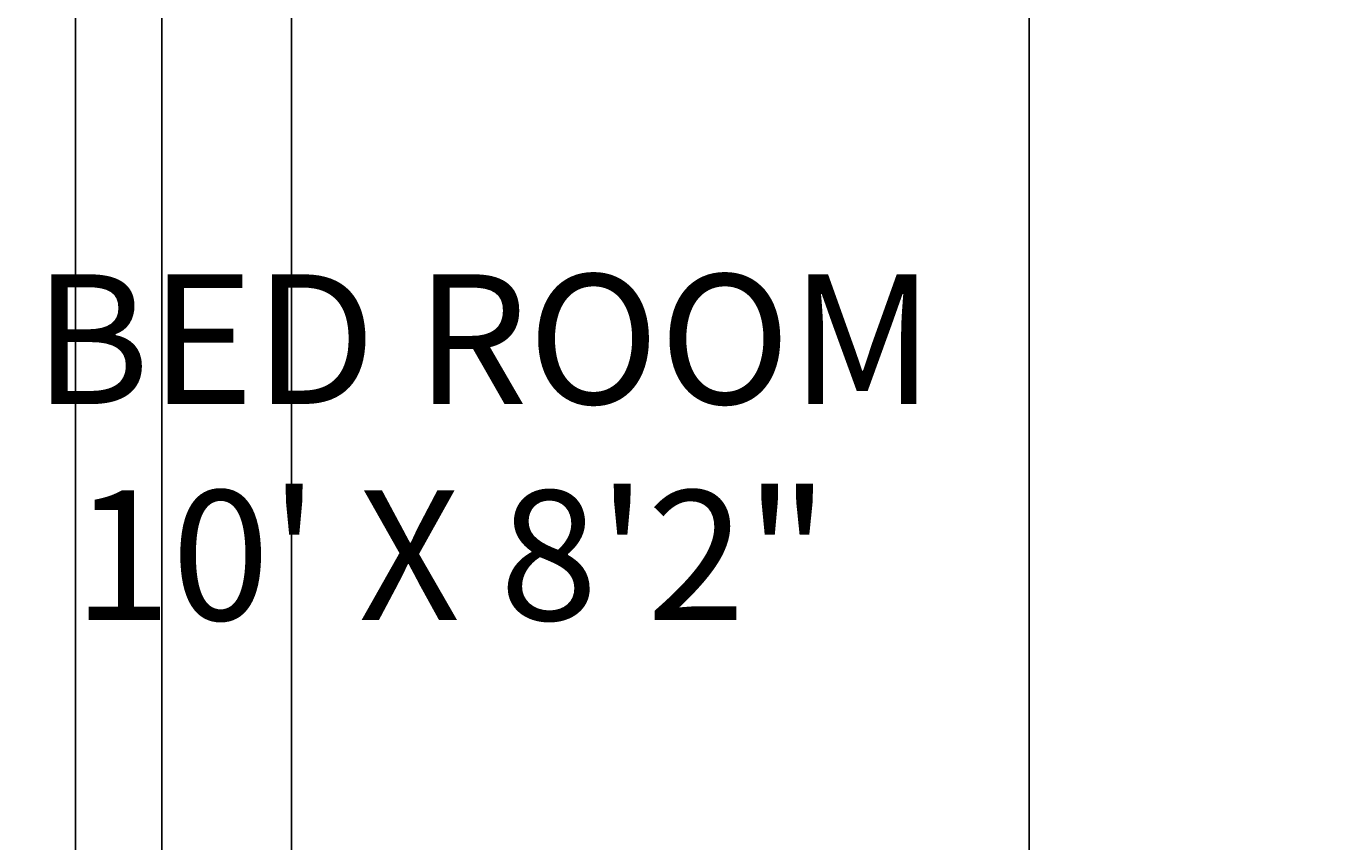
# Model space of a CAD drawing. Units: inches. Extents: x 37 to 824, y -700 to 234.
# Tile 55 of 77: x 204 to 264, y 122 to 160. Entities that reach past the tile are written whole.
import ezdxf

# ---------------------------------------------------------------- set-up
doc = ezdxf.new("R2010")
doc.units = ezdxf.units.IN
doc.header["$MEASUREMENT"] = 0
doc.layers.add('A-ANNO-DIMS', color=2, linetype='Continuous', lineweight=18)
doc.layers.add('A-AREA-IDEN', color=3, linetype='Continuous', lineweight=18)
doc.styles.get("Standard").update_dxf_attribs({"font": 'arial.ttf'})
doc.dimstyles.get("Standard").update_dxf_attribs({"dimtxt": 0.18, "dimasz": 0.18, "dimexe": 0.18, "dimexo": 0.0625, "dimgap": 0.09, "dimtad": 0, "dimtih": 1, "dimtoh": 1, "dimdec": 1, "dimzin": 0, "dimdsep": 46, "dimlunit": 4, "dimtxsty": 'Standard', "dimcen": 0.09, "dimadec": 0, "dimazin": 0, "dimtfac": 1, "dimtdec": 1, "dimtofl": 0, "dimtmove": 0, "dimatfit": 3, "dimfxl": 1, "dimtolj": 1, "dimtzin": 0, "dimarcsym": 0})

# ---------------------------------------------------------------- blocks, each defined once
blk = doc.blocks.new('*D72')
at = {"layer": 'A-ANNO-DIMS', "color": 0, "lineweight": -2, "ltscale": 0.5, "transparency": 16777216}
for p, q in [((170.077, 84.153), (170.077, 234.17)), ((250.19, 84.153), (250.19, 234.17)), ((170.257, 233.99), (209.804, 233.99)), ((250.01, 233.99), (210.463, 233.99))]:
    blk.add_line(p, q, dxfattribs=at)
at = {"layer": 'A-ANNO-DIMS', "color": 0, "ltscale": 0.5, "transparency": 16777216}
for points in [[(170.257, 234.02), (170.257, 233.96), (170.077, 233.99)], [(250.01, 234.02), (250.01, 233.96), (250.19, 233.99)]]:
    blk.add_solid(points, dxfattribs=at)
at = {"layer": 'Defpoints', "color": 0, "ltscale": 0.5, "transparency": 16777216}
for p in [(250.19, 233.99), (170.077, 84.09), (250.19, 84.09)]:
    blk.add_point(p, dxfattribs=at)
at = {"layer": 'A-ANNO-DIMS', "color": 0, "ltscale": 0.5, "transparency": 16777216, "insert": (210.133, 233.99), "char_height": 0.18, "attachment_point": 5}
blk.add_mtext('\\A1;6\'-8"', dxfattribs=at)
blk = doc.blocks.new('*D73')
at = {"layer": 'A-ANNO-DIMS', "color": 0, "lineweight": -2, "ltscale": 0.5, "transparency": 16777216}
for p, q in [((250.19, 84.153), (250.19, 234.17)), ((290.077, 81.153), (290.077, 234.17)), ((250.37, 233.99), (269.804, 233.99)), ((289.897, 233.99), (270.463, 233.99))]:
    blk.add_line(p, q, dxfattribs=at)
at = {"layer": 'A-ANNO-DIMS', "color": 0, "ltscale": 0.5, "transparency": 16777216}
for points in [[(250.37, 234.02), (250.37, 233.96), (250.19, 233.99)], [(289.897, 234.02), (289.897, 233.96), (290.077, 233.99)]]:
    blk.add_solid(points, dxfattribs=at)
at = {"layer": 'Defpoints', "color": 0, "ltscale": 0.5, "transparency": 16777216}
for p in [(290.077, 233.99), (250.19, 84.09), (290.077, 81.09)]:
    blk.add_point(p, dxfattribs=at)
at = {"layer": 'A-ANNO-DIMS', "color": 0, "ltscale": 0.5, "transparency": 16777216, "insert": (270.133, 233.99), "char_height": 0.18, "attachment_point": 5}
blk.add_mtext('\\A1;3\'-4"', dxfattribs=at)
blk = doc.blocks.new('*D84')
at = {"layer": 'A-ANNO-DIMS', "color": 0, "lineweight": -2, "ltscale": 0.5, "transparency": 16777216}
for p, q in [((170.077, -265.847), (170.077, 234.17)), ((210.077, -265.847), (210.077, 234.17)), ((170.257, 233.99), (189.748, 233.99)), ((209.897, 233.99), (190.406, 233.99))]:
    blk.add_line(p, q, dxfattribs=at)
at = {"layer": 'A-ANNO-DIMS', "color": 0, "ltscale": 0.5, "transparency": 16777216}
for points in [[(170.257, 234.02), (170.257, 233.96), (170.077, 233.99)], [(209.897, 234.02), (209.897, 233.96), (210.077, 233.99)]]:
    blk.add_solid(points, dxfattribs=at)
at = {"layer": 'Defpoints', "color": 0, "ltscale": 0.5, "transparency": 16777216}
for p in [(210.077, 233.99), (170.077, -265.91), (210.077, -265.91)]:
    blk.add_point(p, dxfattribs=at)
at = {"layer": 'A-ANNO-DIMS', "color": 0, "ltscale": 0.5, "transparency": 16777216, "insert": (190.077, 233.99), "char_height": 0.18, "attachment_point": 5}
blk.add_mtext('\\A1;3\'-4"', dxfattribs=at)
blk = doc.blocks.new('*D85')
at = {"layer": 'A-ANNO-DIMS', "color": 0, "lineweight": -2, "ltscale": 0.5, "transparency": 16777216}
for p, q in [((170.077, -356.847), (170.077, 234.17)), ((206.077, -356.847), (206.077, 234.17)), ((170.257, 233.99), (187.748, 233.99)), ((205.897, 233.99), (188.406, 233.99))]:
    blk.add_line(p, q, dxfattribs=at)
at = {"layer": 'A-ANNO-DIMS', "color": 0, "ltscale": 0.5, "transparency": 16777216}
for points in [[(170.257, 234.02), (170.257, 233.96), (170.077, 233.99)], [(205.897, 234.02), (205.897, 233.96), (206.077, 233.99)]]:
    blk.add_solid(points, dxfattribs=at)
at = {"layer": 'Defpoints', "color": 0, "ltscale": 0.5, "transparency": 16777216}
for p in [(206.077, 233.99), (170.077, -356.91), (206.077, -356.91)]:
    blk.add_point(p, dxfattribs=at)
at = {"layer": 'A-ANNO-DIMS', "color": 0, "ltscale": 0.5, "transparency": 16777216, "insert": (188.077, 233.99), "char_height": 0.18, "attachment_point": 5}
blk.add_mtext('\\A1;3\'-0"', dxfattribs=at)
blk = doc.blocks.new('*D86')
at = {"layer": 'A-ANNO-DIMS', "color": 0, "lineweight": -2, "ltscale": 0.5, "transparency": 16777216}
for p, q in [((206.077, -356.847), (206.077, 234.17)), ((216.077, -356.847), (216.077, 234.17)), ((206.257, 233.99), (210.678, 233.99)), ((215.897, 233.99), (211.476, 233.99))]:
    blk.add_line(p, q, dxfattribs=at)
at = {"layer": 'A-ANNO-DIMS', "color": 0, "ltscale": 0.5, "transparency": 16777216}
for points in [[(206.257, 234.02), (206.257, 233.96), (206.077, 233.99)], [(215.897, 234.02), (215.897, 233.96), (216.077, 233.99)]]:
    blk.add_solid(points, dxfattribs=at)
at = {"layer": 'Defpoints', "color": 0, "ltscale": 0.5, "transparency": 16777216}
for p in [(216.077, 233.99), (206.077, -356.91), (216.077, -356.91)]:
    blk.add_point(p, dxfattribs=at)
at = {"layer": 'A-ANNO-DIMS', "color": 0, "ltscale": 0.5, "transparency": 16777216, "insert": (211.077, 233.99), "char_height": 0.18, "attachment_point": 5}
blk.add_mtext('\\A1;0\'-10"', dxfattribs=at)
blk = doc.blocks.new('*D87')
at = {"layer": 'A-ANNO-DIMS', "color": 0, "lineweight": -2, "ltscale": 0.5, "transparency": 16777216}
for p, q in [((216.077, -356.847), (216.077, 234.17)), ((296.077, -356.847), (296.077, 234.17)), ((216.257, 233.99), (255.747, 233.99)), ((295.897, 233.99), (256.407, 233.99))]:
    blk.add_line(p, q, dxfattribs=at)
at = {"layer": 'A-ANNO-DIMS', "color": 0, "ltscale": 0.5, "transparency": 16777216}
for points in [[(216.257, 234.02), (216.257, 233.96), (216.077, 233.99)], [(295.897, 234.02), (295.897, 233.96), (296.077, 233.99)]]:
    blk.add_solid(points, dxfattribs=at)
at = {"layer": 'Defpoints', "color": 0, "ltscale": 0.5, "transparency": 16777216}
for p in [(296.077, 233.99), (216.077, -356.91), (296.077, -356.91)]:
    blk.add_point(p, dxfattribs=at)
at = {"layer": 'A-ANNO-DIMS', "color": 0, "ltscale": 0.5, "transparency": 16777216, "insert": (256.077, 233.99), "char_height": 0.18, "attachment_point": 5}
blk.add_mtext('\\A1;6\'-8"', dxfattribs=at)

msp = doc.modelspace()

# ---------------------------------------------------------------- texts
at = {"layer": 'A-AREA-IDEN', "insert": (204.143, 148.167), "char_height": 6, "attachment_point": 1}
msp.add_mtext_dynamic_manual_height_columns('BED ROOM\\P 10\' X 8\'2"', width=88.32168, gutter_width=1, heights=[0], dxfattribs=at)

# ---------------------------------------------------------------- dimensions: what is measured, and where the dimension line sits
at = {"layer": 'A-ANNO-DIMS', "ltscale": 0.5}
for base, p1, p2, picture, middle in [((250.19, 233.99), (170.077, 84.09), (250.19, 84.09), '*D72', (210.133, 233.99)), ((210.077, 233.99), (170.077, -265.91), (210.077, -265.91), '*D84', (190.077, 233.99)), ((206.077, 233.99), (170.077, -356.91), (206.077, -356.91), '*D85', (188.077, 233.99)), ((216.077, 233.99), (206.077, -356.91), (216.077, -356.91), '*D86', (211.077, 233.99)), ((296.077, 233.99), (216.077, -356.91), (296.077, -356.91), '*D87', (256.077, 233.99)), ((290.077, 233.99), (250.19, 84.09), (290.077, 81.09), '*D73', (270.133, 233.99))]:
    dim = msp.add_linear_dim(base=base, p1=p1, p2=p2, dimstyle='Standard', override={"dimdec": 1, "dimlfac": 1, "dimrnd": 0, "dimzin": 1, "dimdsep": 46, "dimlunit": 4, "dimfrac": 2}, dxfattribs=at)
    dim.commit()
    dim.dimension.update_dxf_attribs({"geometry": picture, "text_midpoint": middle})

doc.saveas('drawing.dxf')
